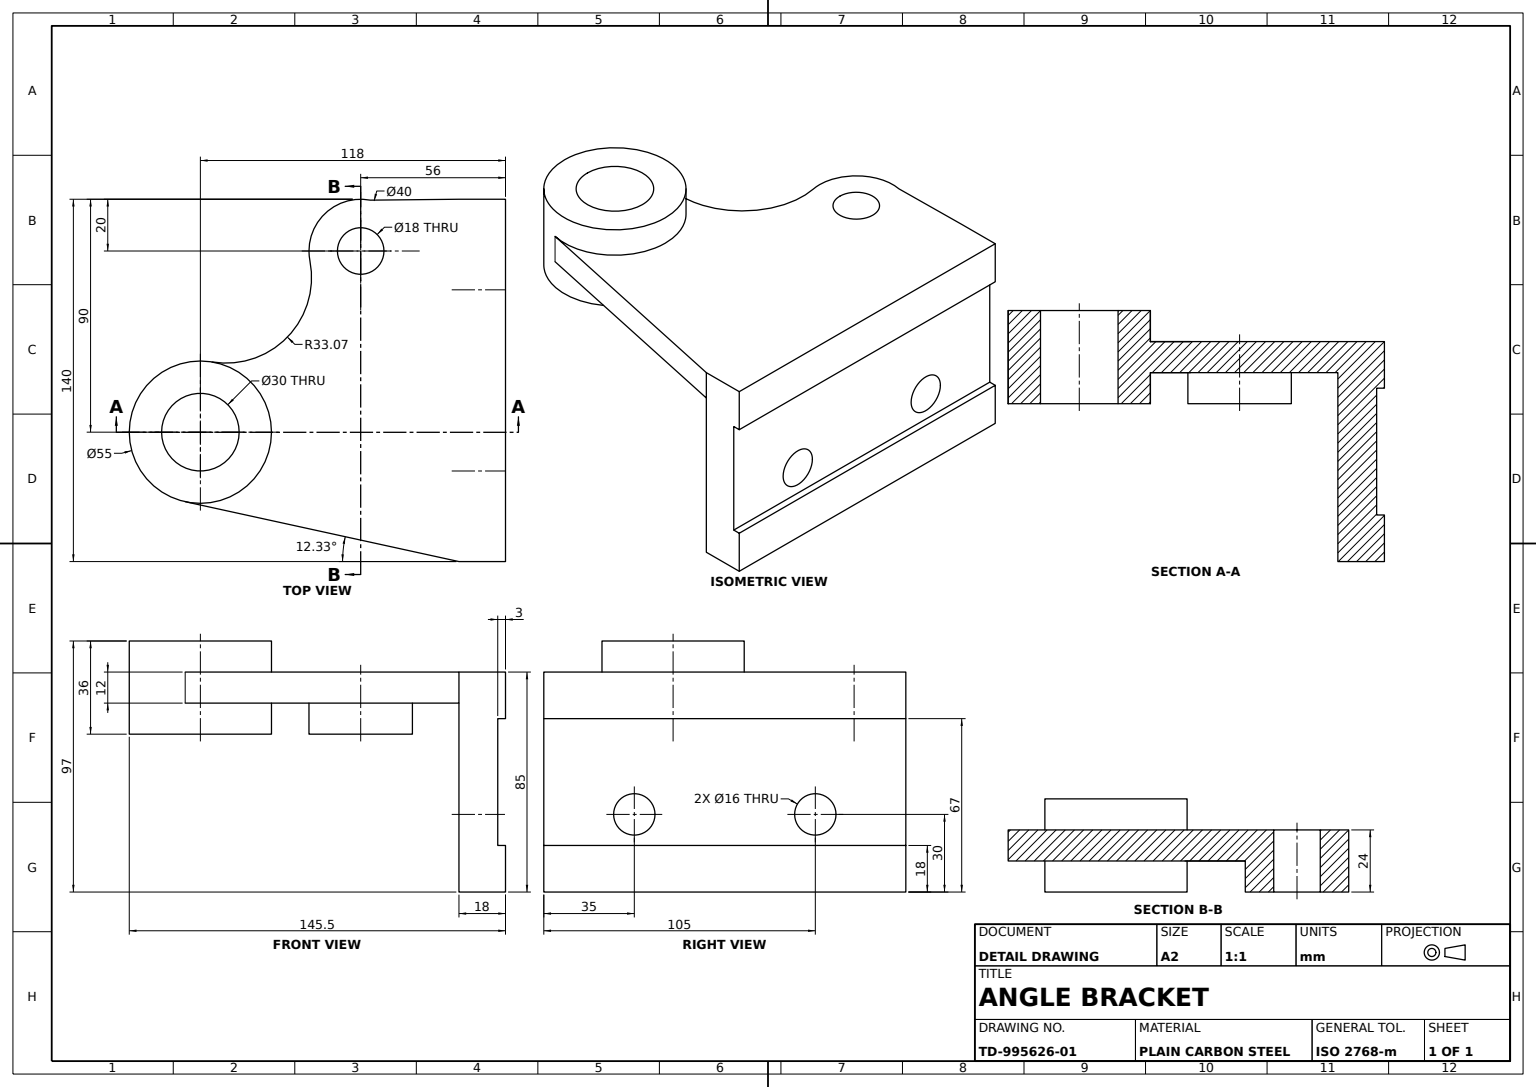
SolidWorks part; units mm, degrees
material "Plain Carbon Steel"
ref_plane "Front Plane" through (0, 0, 0) normal (0, 0, 1) x (1, 0, 0)
ref_plane "Top Plane" through (0, 0, 0) normal (0, 1, 0) x (1, 0, 0)
ref_plane "Right Plane" through (0, 0, 0) normal (1, 0, 0) x (0, 0, -1)
sketch "Base Plate Sketch" plane through (0, 0, 0) normal (0, 0, 1) x (1, 0, 0)
  line L0 (0, 0) -> (140, 0)
  line L1 (140, 0) -> (140, -85)
  line L2 (140, -85) -> (0, -85)
  line L3 (0, -85) -> (0, 0)
  dimension "D1" = 140
  dimension "D2" = 85
extrude "Base Plate 18mm" add sketch "Base Plate Sketch" along normal blind 18
sketch "Plate Profile Cut Sketch" plane through (0, 0, 0) normal (-1, 0, 0) x (0, 0, 1)
  line L1 (18, -85) -> (0, -85) construction
  line L3 (3, -18) -> (0, -18)
  line L4 (0, 0) -> (0, -85) construction
  line L9 (3, -67) -> (0, -67)
  line L10 (3, -18) -> (3, -67)
  line L11 (0, -18) -> (0, -67)
  dimension "D1" = 3
  dimension "D2" = 18
  dimension "D3" = 67
extrude "Plate Profile Cut" cut sketch "Plate Profile Cut Sketch" against normal blind 140
sketch "Notch 16x16 Sketch" plane through (0, 0, 18) normal (0, 0, 1) x (1, 0, 0)
  line L0 (0, 0) -> (0, -85) construction
  line L1 (0, -85) -> (140, -85) construction
  circle A0 centre (35, -55) radius 8
  circle A1 centre (105, -55) radius 8
  dimension "D1" = 16
  dimension "D2" = 16
  dimension "D3" = 16
  dimension "D4" = 35
  dimension "D5" = 105
  dimension "D6" = 30
extrude "Notch 16x16" cut sketch "Notch 16x16 Sketch" against normal blind 140
sketch "Small Eye Boss Ø40 Sketch" plane through (0, 0, 0) normal (0, 1, 0) x (1, 0, 0)
  line L0 (0, -18) -> (0, 0) construction
  line L1 (140, 0) -> (0, 0) construction
  circle A0 centre (20, -56) radius 20
  dimension "D1" = 40
  dimension "D2" = 40
  dimension "D3" = 20
  dimension "D4" = 56
extrude "Small Eye Boss Ø40" add sketch "Small Eye Boss Ø40 Sketch" against normal blind 12 separate body
sketch "Large Eye Boss Ø55 Sketch" plane through (0, 0, 0) normal (0, 1, 0) x (1, 0, 0)
  line L0 (0, -18) -> (0, 0) construction
  line L1 (140, 0) -> (0, 0) construction
  circle A0 centre (90, -118) radius 27.5
  dimension "D1" = 55
  dimension "D2" = 55
  dimension "D3" = 90
  dimension "D4" = 118
extrude "Large Eye Boss Ø55" add sketch "Large Eye Boss Ø55 Sketch" against normal blind 12 separate body
sketch "Eye Link Web Sketch" plane through (0, 0, 0) normal (0, 1, 0) x (1, 0, 0)
  line L0 (0, -18) -> (0.3536, -52.256)
  line L1 (140, -18) -> (116.8661, -123.8705)
  line L2 (0, -18) -> (140, -18)
  line L3 (0, -18) -> (0, 0) construction
  circle A0 centre (20, -56) radius 20 construction
  circle A1 centre (90, -118) radius 27.5 construction
  arc A2 (23.8632, -75.6234) -> (62.8721, -113.4913) centre (30.2507, -108.0695) cw
  arc A3 (23.8632, -75.6234) -> (0.3536, -52.256) centre (20, -56) ccw
  arc A5 (116.8661, -123.8705) -> (62.8721, -113.4913) centre (90, -118) ccw
  dimension "D1" = 33.0689
  dimension "D2" = 40
  dimension "D3" = 55
  dimension "D4" = 27.5
  dimension "D5" = 33.0689
  dimension "D6" = 0.3536
  dimension "D7" = 62.8721
extrude "Eye Link Web" add sketch "Eye Link Web Sketch" against normal blind 12
sketch "Large Eye Cap Ø55 Sketch" plane through (0, 0, 0) normal (0, 1, 0) x (1, 0, 0)
  circle A0 centre (90, -118) radius 27.5
  dimension "D1" = 55
  dimension "D2" = 55
extrude "Large Eye Cap Ø55" add sketch "Large Eye Cap Ø55 Sketch" along normal blind 12
sketch "Large Eye Extension Ø55 Sketch" plane through (0, -12, 0) normal (0, -1, 0) x (1, 0, 0)
  circle A0 centre (90, 118) radius 27.5
  dimension "D1" = 55
  dimension "D2" = 55
extrude "Large Eye Extension Ø55" add sketch "Large Eye Extension Ø55 Sketch" along normal blind 12
sketch "Small Eye Extension Ø40 Sketch" plane through (0, -12, 0) normal (0, -1, 0) x (1, 0, 0)
  circle A0 centre (20, 56) radius 20
  dimension "D1" = 40
  dimension "D2" = 40
extrude "Small Eye Extension Ø40" add sketch "Small Eye Extension Ø40 Sketch" along normal blind 12
sketch "Large Eye Bore Ø30 Sketch" plane through (0, -24, 0) normal (0, -1, 0) x (1, 0, 0)
  circle A0 centre (90, 118) radius 15
  dimension "D1" = 30
  dimension "D2" = 30
extrude "Large Eye Bore Ø30" cut sketch "Large Eye Bore Ø30 Sketch" against normal blind 36
sketch "Small Eye Bore Ø18 Sketch" plane through (0, -24, 0) normal (0, -1, 0) x (1, 0, 0)
  circle A0 centre (20, 56) radius 9
  dimension "D1" = 18
  dimension "D2" = 18
extrude "Small Eye Bore Ø18" cut sketch "Small Eye Bore Ø18 Sketch" against normal blind 24
